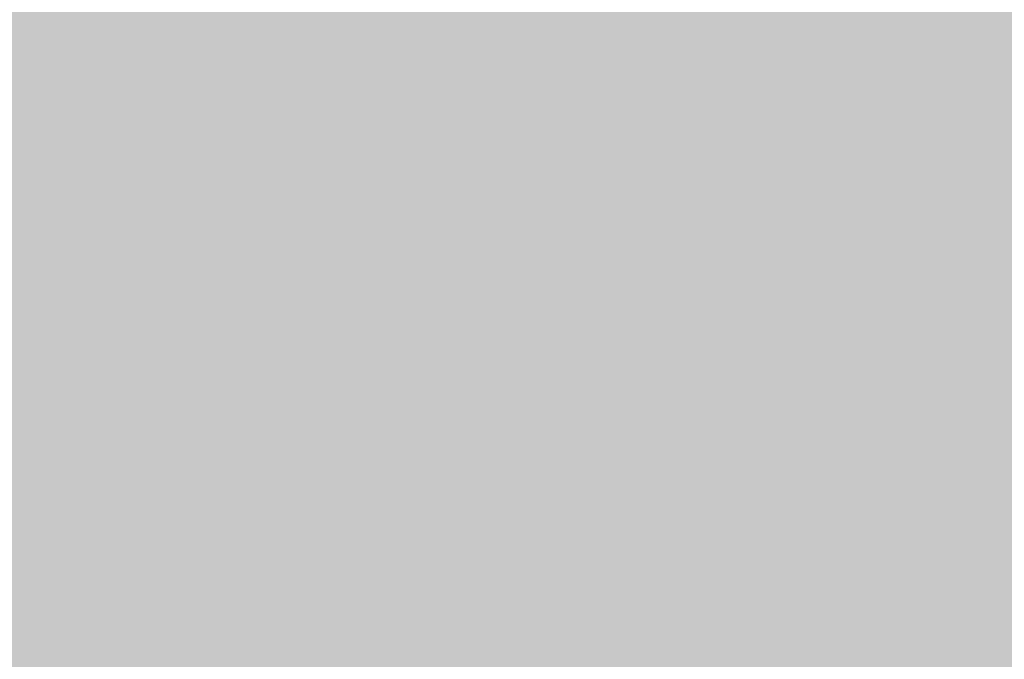
# Model space of a CAD drawing. Units: millimetres. Extents: x 0 to 2267, y 0 to 1823.
# Tile 135 of 256: x 1675 to 1760, y 1160 to 1216. Entities that reach past the tile are written whole.
import ezdxf

# ---------------------------------------------------------------- set-up
doc = ezdxf.new("R2010")
doc.units = ezdxf.units.MM
doc.header["$MEASUREMENT"] = 0
doc.layers.add('M-HATC', color=252, linetype='Continuous', lineweight=18)

msp = doc.modelspace()

# ---------------------------------------------------------------- hatches: boundary and pattern name
at = {"layer": 'M-HATC'}
h = msp.add_hatch(color=256, dxfattribs=at)
h.dxf.hatch_style = 1
h.paths.add_polyline_path([(2055.771, 1603.062), (1381.087, 1603.062), (1381.087, 1598.062), (2055.771, 1598.062)])
h.paths.add_polyline_path([(2055.771, 1598.062), (1381.087, 1598.062), (1381.087, 1593.062), (2055.771, 1593.062)])
h.paths.add_polyline_path([(2051.307, 1536.761), (1385.55, 1536.761), (1385.55, 1526.761), (1387.55, 1526.761), (1388.537, 1525.053), (1385.332, 1521.233), (1385.332, 1521.223), (2050.254, 1522.749), (2048.321, 1525.053), (2049.307, 1526.761), (2051.307, 1526.761)])
edge = h.paths.add_edge_path()
edge.add_arc((1847.535, 1379.149), 135, 222.60306, 222.89085, ccw=False)
edge.add_line((1748.166, 1287.766), (1683.092, 1287.766))
edge.add_arc((1583.724, 1379.149), 135, 317.10915, 317.39694, ccw=False)
edge.add_arc((1678.969, 1290.671), 5, 222.89085, 317.10915, ccw=False)
edge.add_arc((1774.213, 1379.149), 135, 222.60306, 222.89085, ccw=False)
edge.add_line((1674.845, 1287.766), (1609.771, 1287.766))
edge.add_arc((1510.403, 1379.149), 135, 317.10915, 317.39694, ccw=False)
edge.add_arc((1605.647, 1290.671), 5, 222.89085, 317.10915, ccw=False)
edge.add_arc((1700.892, 1379.149), 135, 222.60306, 222.89085, ccw=False)
edge.add_line((1601.524, 1287.766), (1536.45, 1287.766))
edge.add_arc((1437.081, 1379.149), 135, 317.10915, 317.39694, ccw=False)
edge.add_arc((1532.326, 1290.671), 5, 222.89085, 317.10915, ccw=False)
edge.add_arc((1627.571, 1379.149), 135, 222.60306, 222.89085, ccw=False)
edge.add_line((1528.203, 1287.766), (1505.929, 1287.766))
edge.add_spline(control_points=[(1505.929, 1287.766), (1504.262, 1287.766), (1504.262, 1282.766), (1505.929, 1282.766)], knot_values=[0, 0, 0, 0, 5, 5, 5, 5], degree=3, periodic=0)
edge.add_line((1505.929, 1282.766), (1930.929, 1282.766))
edge.add_spline(control_points=[(1930.929, 1282.766), (1932.596, 1282.766), (1932.596, 1287.766), (1930.929, 1287.766)], knot_values=[0, 0, 0, 0, 5, 5, 5, 5], degree=3, periodic=0)
edge.add_line((1930.929, 1287.766), (1903.056, 1287.766))
edge.add_arc((1803.688, 1379.149), 135, 317.10915, 317.39694, ccw=False)
edge.add_arc((1898.932, 1290.671), 5, 222.89085, 317.10915, ccw=False)
edge.add_arc((1994.177, 1379.149), 135, 222.60306, 222.89085, ccw=False)
edge.add_line((1894.809, 1287.766), (1829.735, 1287.766))
edge.add_arc((1730.366, 1379.149), 135, 317.10915, 317.39694, ccw=False)
edge.add_arc((1825.611, 1290.671), 5, 222.89085, 317.10915, ccw=False)
edge.add_arc((1920.856, 1379.149), 135, 222.60306, 222.89085, ccw=False)
edge.add_line((1821.487, 1287.766), (1756.413, 1287.766))
edge.add_arc((1657.045, 1379.149), 135, 317.10915, 317.39694, ccw=False)
edge.add_arc((1752.29, 1290.671), 5, 222.89085, 317.10915, ccw=False)
edge = h.paths.add_edge_path()
edge.add_spline(control_points=[(1843.429, 1227.247), (1845.096, 1227.247), (1845.096, 1232.247), (1843.429, 1232.247)], knot_values=[0, 0, 0, 0, 5, 5, 5, 5], degree=3, periodic=0)
edge.add_line((1843.429, 1232.247), (1593.429, 1232.247))
edge.add_spline(control_points=[(1593.429, 1232.247), (1591.762, 1232.247), (1591.762, 1227.247), (1593.429, 1227.247)], knot_values=[0, 0, 0, 0, 5, 5, 5, 5], degree=3, periodic=0)
edge.add_line((1593.429, 1227.247), (1843.429, 1227.247))
h.paths.add_polyline_path([(1905.929, 1127.417), (1530.929, 1127.417, 0.414214), (1520.929, 1117.417), (1530.929, 1117.417), (1915.929, 1117.417, 0.414214)])
edge = h.paths.add_edge_path()
edge.add_arc((1397.086, 1498.408), 12.73, 90.78215, 190.87871, ccw=False)
edge.add_line((1396.912, 1511.136), (1428.01, 1511.349))
edge.add_line((1428.01, 1511.349), (1433.01, 1511.349))
edge.add_line((1433.01, 1511.349), (1434.439, 1511.349))
edge.add_arc((1419.474, 1498.08), 20, 41.561, 74.08211)
edge.add_line((1424.959, 1517.314), (1399.935, 1517.256))
edge.add_spline(control_points=[(1399.931, 1517.256), (1399.884, 1517.213), (1399.833, 1517.169), (1399.777, 1517.124)], knot_values=[11.567499, 11.567499, 11.567499, 11.567499, 11.814249, 11.814249, 11.814249, 11.814249], degree=3, periodic=0)
edge.add_spline(control_points=[(1399.633, 1517.01), (1399.583, 1516.972), (1399.531, 1516.934), (1399.476, 1516.895)], knot_values=[11.167718, 11.167718, 11.167718, 11.167718, 11.365188, 11.365188, 11.365188, 11.365188], degree=3, periodic=0)
edge.add_spline(control_points=[(1399.34, 1516.8), (1399.151, 1516.672), (1398.938, 1516.538), (1398.704, 1516.399)], knot_values=[10.376405, 10.376405, 10.376405, 10.376405, 11.00994, 11.00994, 11.00994, 11.00994], degree=3, periodic=0)
edge.add_spline(control_points=[(1398.657, 1516.372), (1398.579, 1516.326), (1398.498, 1516.28), (1398.415, 1516.233)], knot_values=[10.125175, 10.125175, 10.125175, 10.125175, 10.334406, 10.334406, 10.334406, 10.334406], degree=3, periodic=0)
edge.add_spline(control_points=[(1398.264, 1516.149), (1398.196, 1516.111), (1398.126, 1516.073), (1398.055, 1516.035)], knot_values=[9.832246, 9.832246, 9.832246, 9.832246, 9.999658, 9.999658, 9.999658, 9.999658], degree=3, periodic=0)
edge.add_spline(control_points=[(1397.999, 1516.005), (1397.731, 1515.862), (1397.446, 1515.717), (1397.147, 1515.571)], knot_values=[9.161808, 9.161808, 9.161808, 9.161808, 9.787769, 9.787769, 9.787769, 9.787769], degree=3, periodic=0)
edge.add_spline(control_points=[(1397.147, 1515.571), (1396.842, 1515.423), (1396.522, 1515.274), (1396.191, 1515.126)], knot_values=[8.524455, 8.524455, 8.524455, 8.524455, 9.161808, 9.161808, 9.161808, 9.161808], degree=3, periodic=0)
edge.add_spline(control_points=[(1396.078, 1515.076), (1395.985, 1515.035), (1395.892, 1514.994), (1395.798, 1514.953)], knot_values=[8.275193, 8.275193, 8.275193, 8.275193, 8.451726, 8.451726, 8.451726, 8.451726], degree=3, periodic=0)
edge.add_spline(control_points=[(1395.602, 1514.869), (1395.5, 1514.826), (1395.397, 1514.782), (1395.293, 1514.739)], knot_values=[7.962917, 7.962917, 7.962917, 7.962917, 8.152764, 8.152764, 8.152764, 8.152764], degree=3, periodic=0)
edge.add_spline(control_points=[(1395.212, 1514.706), (1394.828, 1514.547), (1394.435, 1514.393), (1394.036, 1514.244)], knot_values=[7.21254, 7.21254, 7.21254, 7.21254, 7.913148, 7.913148, 7.913148, 7.913148], degree=3, periodic=0)
edge.add_spline(control_points=[(1394.036, 1514.244), (1393.708, 1514.121), (1393.375, 1514.003), (1393.043, 1513.889)], knot_values=[6.633733, 6.633733, 6.633733, 6.633733, 7.21254, 7.21254, 7.21254, 7.21254], degree=3, periodic=0)
edge.add_spline(control_points=[(1392.821, 1513.815), (1392.72, 1513.781), (1392.618, 1513.748), (1392.517, 1513.715)], knot_values=[6.328796, 6.328796, 6.328796, 6.328796, 6.505493, 6.505493, 6.505493, 6.505493], degree=3, periodic=0)
edge.add_spline(control_points=[(1392.517, 1513.715), (1392.319, 1513.652), (1392.121, 1513.59), (1391.924, 1513.531)], knot_values=[5.984605, 5.984605, 5.984605, 5.984605, 6.328796, 6.328796, 6.328796, 6.328796], degree=3, periodic=0)
edge.add_spline(control_points=[(1391.792, 1513.491), (1391.312, 1513.35), (1390.838, 1513.224), (1390.378, 1513.117)], knot_values=[5.066697, 5.066697, 5.066697, 5.066697, 5.907055, 5.907055, 5.907055, 5.907055], degree=3, periodic=0)
edge.add_spline(control_points=[(1390.378, 1513.117), (1390.18, 1513.071), (1389.984, 1513.028), (1389.791, 1512.99)], knot_values=[4.70367, 4.70367, 4.70367, 4.70367, 5.066695, 5.066695, 5.066695, 5.066695], degree=3, periodic=0)
edge.add_spline(control_points=[(1389.422, 1512.92), (1389.246, 1512.889), (1389.073, 1512.862), (1388.904, 1512.838)], knot_values=[4.130571, 4.130571, 4.130571, 4.130571, 4.469816, 4.469816, 4.469816, 4.469816], degree=3, periodic=0)
edge.add_spline(control_points=[(1388.904, 1512.838), (1388.591, 1512.795), (1388.291, 1512.764), (1388.007, 1512.749)], knot_values=[3.504031, 3.504031, 3.504031, 3.504031, 4.130571, 4.130571, 4.130571, 4.130571], degree=3, periodic=0)
edge.add_spline(control_points=[(1387.936, 1512.746), (1387.854, 1512.742), (1387.773, 1512.74), (1387.694, 1512.739)], knot_values=[3.268866, 3.268866, 3.268866, 3.268866, 3.451164, 3.451164, 3.451164, 3.451164], degree=3, periodic=0)
edge.add_spline(control_points=[(1387.335, 1512.744), (1387.208, 1512.75), (1387.085, 1512.76), (1386.967, 1512.774)], knot_values=[2.670686, 2.670686, 2.670686, 2.670686, 2.984, 2.984, 2.984, 2.984], degree=3, periodic=0)
edge.add_spline(control_points=[(1386.833, 1512.792), (1386.821, 1512.794), (1386.809, 1512.796), (1386.797, 1512.798)], knot_values=[2.516981, 2.516981, 2.516981, 2.516981, 2.549528, 2.549528, 2.549528, 2.549528], degree=3, periodic=0)
edge.add_spline(control_points=[(1386.453, 1512.873), (1386.426, 1512.881), (1386.399, 1512.889), (1386.373, 1512.897)], knot_values=[2.095869, 2.095869, 2.095869, 2.095869, 2.17941, 2.17941, 2.17941, 2.17941], degree=3, periodic=0)
edge.add_spline(control_points=[(1386.069, 1513.019), (1386.063, 1513.022), (1386.058, 1513.025), (1386.052, 1513.028)], knot_values=[1.72453, 1.72453, 1.72453, 1.72453, 1.745933, 1.745933, 1.745933, 1.745933], degree=3, periodic=0)
edge.add_arc((1399.474, 1498.08), 20, 131.82432, 180)
edge.add_arc((1630.334, 1505.548), 250.971, 181.70518, 236.42798)
edge.add_arc((1605.34, 1483.304), 218.782, 238.66083, 243.34961)
edge.add_arc((1647.091, 1510.359), 262.899, 183.12984, 237.85344, ccw=False)
h.paths.add_polyline_path([(1406.537, 1391.964, 0.149382), (1491.551, 1296.442, -0.129517)], flags=17)
edge = h.paths.add_edge_path()
edge.add_arc((2037.384, 1498.08), 20, 0, 48.26587)
edge.add_spline(control_points=[(2050.697, 1513.005), (2050.651, 1512.985), (2050.603, 1512.966), (2050.554, 1512.948)], knot_values=[1.835652, 1.835652, 1.835652, 1.835652, 2.000781, 2.000781, 2.000781, 2.000781], degree=3, periodic=0)
edge.add_spline(control_points=[(2050.462, 1512.917), (2050.479, 1512.922), (2050.496, 1512.928), (2050.513, 1512.934)], knot_values=[2.045477, 2.045477, 2.045477, 2.045477, 2.101389, 2.101389, 2.101389, 2.101389], degree=3, periodic=0)
edge.add_spline(control_points=[(2050.129, 1512.834), (2050.198, 1512.847), (2050.266, 1512.862), (2050.331, 1512.879)], knot_values=[2.237629, 2.237629, 2.237629, 2.237629, 2.435841, 2.435841, 2.435841, 2.435841], degree=3, periodic=0)
edge.add_spline(control_points=[(2050.095, 1512.828), (2050.106, 1512.83), (2050.118, 1512.832), (2050.129, 1512.834)], knot_values=[2.435841, 2.435841, 2.435841, 2.435841, 2.468321, 2.468321, 2.468321, 2.468321], degree=3, periodic=0)
edge.add_spline(control_points=[(2049.784, 1512.785), (2049.855, 1512.792), (2049.924, 1512.801), (2049.992, 1512.811)], knot_values=[2.563852, 2.563852, 2.563852, 2.563852, 2.748541, 2.748541, 2.748541, 2.748541], degree=3, periodic=0)
edge.add_spline(control_points=[(2049.405, 1512.762), (2049.536, 1512.765), (2049.663, 1512.773), (2049.784, 1512.785)], knot_values=[2.748541, 2.748541, 2.748541, 2.748541, 3.064882, 3.064882, 3.064882, 3.064882], degree=3, periodic=0)
edge.add_spline(control_points=[(2049.17, 1512.76), (2049.234, 1512.759), (2049.297, 1512.759), (2049.358, 1512.761)], knot_values=[3.102309, 3.102309, 3.102309, 3.102309, 3.2503, 3.2503, 3.2503, 3.2503], degree=3, periodic=0)
edge.add_spline(control_points=[(2048.857, 1512.769), (2048.964, 1512.764), (2049.068, 1512.761), (2049.17, 1512.76)], knot_values=[3.2503, 3.2503, 3.2503, 3.2503, 3.486069, 3.486069, 3.486069, 3.486069], degree=3, periodic=0)
edge.add_spline(control_points=[(2048.692, 1512.779), (2048.373, 1512.801), (2048.035, 1512.841), (2047.682, 1512.897)], knot_values=[3.606429, 3.606429, 3.606429, 3.606429, 4.2989, 4.2989, 4.2989, 4.2989], degree=3, periodic=0)
edge.add_spline(control_points=[(2047.682, 1512.897), (2047.546, 1512.919), (2047.408, 1512.942), (2047.268, 1512.969)], knot_values=[4.2989, 4.2989, 4.2989, 4.2989, 4.565769, 4.565769, 4.565769, 4.565769], degree=3, periodic=0)
edge.add_spline(control_points=[(2047.268, 1512.969), (2047.145, 1512.991), (2047.021, 1513.016), (2046.895, 1513.042)], knot_values=[4.565769, 4.565769, 4.565769, 4.565769, 4.799971, 4.799971, 4.799971, 4.799971], degree=3, periodic=0)
edge.add_spline(control_points=[(2046.895, 1513.042), (2046.529, 1513.119), (2046.151, 1513.209), (2045.768, 1513.311)], knot_values=[4.799971, 4.799971, 4.799971, 4.799971, 5.483718, 5.483718, 5.483718, 5.483718], degree=3, periodic=0)
edge.add_spline(control_points=[(2045.768, 1513.311), (2045.372, 1513.415), (2044.97, 1513.532), (2044.566, 1513.659)], knot_values=[5.483718, 5.483718, 5.483718, 5.483718, 6.187866, 6.187866, 6.187866, 6.187866], degree=3, periodic=0)
edge.add_spline(control_points=[(2044.566, 1513.659), (2044.415, 1513.706), (2044.263, 1513.755), (2044.112, 1513.805)], knot_values=[6.187866, 6.187866, 6.187866, 6.187866, 6.451551, 6.451551, 6.451551, 6.451551], degree=3, periodic=0)
edge.add_spline(control_points=[(2044.112, 1513.805), (2043.997, 1513.843), (2043.882, 1513.881), (2043.767, 1513.92)], knot_values=[6.451551, 6.451551, 6.451551, 6.451551, 6.651434, 6.651434, 6.651434, 6.651434], degree=3, periodic=0)
edge.add_spline(control_points=[(2043.767, 1513.92), (2043.372, 1514.055), (2042.977, 1514.198), (2042.589, 1514.346)], knot_values=[6.651434, 6.651434, 6.651434, 6.651434, 7.338879, 7.338879, 7.338879, 7.338879], degree=3, periodic=0)
edge.add_spline(control_points=[(2042.589, 1514.346), (2042.164, 1514.507), (2041.746, 1514.675), (2041.341, 1514.846)], knot_values=[7.338879, 7.338879, 7.338879, 7.338879, 8.089209, 8.089209, 8.089209, 8.089209], degree=3, periodic=0)
edge.add_spline(control_points=[(2041.341, 1514.846), (2041.103, 1514.946), (2040.869, 1515.048), (2040.64, 1515.15)], knot_values=[8.089209, 8.089209, 8.089209, 8.089209, 8.529587, 8.529587, 8.529587, 8.529587], degree=3, periodic=0)
edge.add_spline(control_points=[(2040.51, 1515.209), (2040.082, 1515.402), (2039.675, 1515.597), (2039.295, 1515.789)], knot_values=[8.613818, 8.613818, 8.613818, 8.613818, 9.44571, 9.44571, 9.44571, 9.44571], degree=3, periodic=0)
edge.add_spline(control_points=[(2039.295, 1515.789), (2039.062, 1515.907), (2038.839, 1516.025), (2038.629, 1516.14)], knot_values=[9.44571, 9.44571, 9.44571, 9.44571, 9.956404, 9.956404, 9.956404, 9.956404], degree=3, periodic=0)
edge.add_spline(control_points=[(2038.629, 1516.14), (2038.519, 1516.2), (2038.412, 1516.26), (2038.309, 1516.319)], knot_values=[9.956404, 9.956404, 9.956404, 9.956404, 10.223542, 10.223542, 10.223542, 10.223542], degree=3, periodic=0)
edge.add_spline(control_points=[(2038.309, 1516.319), (2038.214, 1516.374), (2038.122, 1516.428), (2038.033, 1516.481)], knot_values=[10.223542, 10.223542, 10.223542, 10.223542, 10.47051, 10.47051, 10.47051, 10.47051], degree=3, periodic=0)
edge.add_spline(control_points=[(2038.033, 1516.481), (2037.786, 1516.63), (2037.564, 1516.773), (2037.372, 1516.909)], knot_values=[10.47051, 10.47051, 10.47051, 10.47051, 11.15767, 11.15767, 11.15767, 11.15767], degree=3, periodic=0)
edge.add_spline(control_points=[(2037.372, 1516.909), (2037.279, 1516.975), (2037.193, 1517.04), (2037.114, 1517.102)], knot_values=[11.15767, 11.15767, 11.15767, 11.15767, 11.49227, 11.49227, 11.49227, 11.49227], degree=3, periodic=0)
edge.add_spline(control_points=[(2036.856, 1517.326), (2036.915, 1517.269), (2036.981, 1517.21), (2037.056, 1517.149)], knot_values=[11.577341, 11.577341, 11.577341, 11.577341, 11.91035, 11.91035, 11.91035, 11.91035], degree=3, periodic=0)
edge.add_spline(control_points=[(2036.807, 1517.375), (2036.823, 1517.359), (2036.839, 1517.342), (2036.856, 1517.326)], knot_values=[11.91035, 11.91035, 11.91035, 11.91035, 12.007402, 12.007402, 12.007402, 12.007402], degree=3, periodic=0)
edge.add_spline(control_points=[(2036.702, 1517.494), (2036.71, 1517.483), (2036.72, 1517.472), (2036.729, 1517.461)], knot_values=[12.184155, 12.184155, 12.184155, 12.184155, 12.255409, 12.255409, 12.255409, 12.255409], degree=3, periodic=0)
edge.add_spline(control_points=[(2036.616, 1517.621), (2036.62, 1517.613), (2036.624, 1517.606), (2036.629, 1517.598)], knot_values=[12.487913, 12.487913, 12.487913, 12.487913, 12.541035, 12.541035, 12.541035, 12.541035], degree=3, periodic=0)
edge.add_spline(control_points=[(2036.563, 1517.786), (2036.564, 1517.779), (2036.564, 1517.773), (2036.565, 1517.766)], knot_values=[12.911761, 12.911761, 12.911761, 12.911761, 12.968286, 12.968286, 12.968286, 12.968286], degree=3, periodic=0)
edge.add_spline(control_points=[(2036.617, 1517.93), (2036.612, 1517.926), (2036.609, 1517.921), (2036.605, 1517.916)], knot_values=[13.382527, 13.382527, 13.382527, 13.382527, 13.433791, 13.433791, 13.433791, 13.433791], degree=3, periodic=0)
edge.add_spline(control_points=[(2036.749, 1518.017), (2036.736, 1518.012), (2036.724, 1518.006), (2036.712, 1518)], knot_values=[13.726299, 13.726299, 13.726299, 13.726299, 13.809928, 13.809928, 13.809928, 13.809928], degree=3, periodic=0)
edge.add_spline(control_points=[(2036.86, 1518.053), (2036.839, 1518.047), (2036.818, 1518.042), (2036.799, 1518.035)], knot_values=[13.910887, 13.910887, 13.910887, 13.910887, 14.02153, 14.02153, 14.02153, 14.02153], degree=3, periodic=0)
edge.add_line((2036.964, 1518.08), (2032.384, 1518.08))
edge.add_line((2032.384, 1518.08), (2027.384, 1518.08))
edge.add_line((2027.384, 1518.08), (2022.384, 1518.08))
edge.add_line((2022.384, 1518.08), (2017.384, 1518.08))
edge.add_arc((2017.384, 1498.08), 20, 90, 138.439)
edge.add_line((2002.419, 1511.349), (2003.848, 1511.349))
edge.add_line((2003.848, 1511.349), (2008.848, 1511.349))
edge.add_line((2008.848, 1511.349), (2039.772, 1511.138))
edge.add_arc((2039.772, 1498.408), 12.73, -10.87871, 90, ccw=False)
edge.add_arc((1789.767, 1510.359), 262.899, 302.14656, 356.87016, ccw=False)
edge.add_arc((1831.518, 1483.304), 218.782, 296.65039, 301.33917)
edge.add_arc((1806.524, 1505.548), 250.971, 303.57202, 358.29482)
h.paths.add_polyline_path([(2030.321, 1391.964, -0.129517), (1945.307, 1296.442, 0.149382)], flags=17)
edge = h.paths.add_edge_path()
edge.add_spline(control_points=[(2037.246, 1518.082), (2037.29, 1518.081), (2037.336, 1518.08), (2037.384, 1518.08)], knot_values=[0.000012, 0.000012, 0.000012, 0.000012, 0.144754, 0.144754, 0.144754, 0.144754], degree=3, periodic=0)
edge.add_line((2037.336, 1518.08), (2037.01, 1518.08))
edge.add_spline(control_points=[(2037.01, 1518.08), (2036.982, 1518.077), (2036.956, 1518.073), (2036.931, 1518.068)], knot_values=[14.13465, 14.13465, 14.13465, 14.13465, 14.247197, 14.247197, 14.247197, 14.247197], degree=3, periodic=0)
edge.add_spline(control_points=[(2036.931, 1518.068), (2036.928, 1518.067), (2036.924, 1518.067), (2036.921, 1518.066)], knot_values=[14.118315, 14.118315, 14.118315, 14.118315, 14.13465, 14.13465, 14.13465, 14.13465], degree=3, periodic=0)
edge.add_spline(control_points=[(2036.921, 1518.066), (2036.912, 1518.064), (2036.903, 1518.063), (2036.895, 1518.061)], knot_values=[14.078086, 14.078086, 14.078086, 14.078086, 14.118315, 14.118315, 14.118315, 14.118315], degree=3, periodic=0)
edge.add_spline(control_points=[(2036.895, 1518.061), (2036.883, 1518.058), (2036.872, 1518.056), (2036.86, 1518.053)], knot_values=[14.02153, 14.02153, 14.02153, 14.02153, 14.078086, 14.078086, 14.078086, 14.078086], degree=3, periodic=0)
edge.add_spline(control_points=[(2036.86, 1518.053), (2036.839, 1518.047), (2036.818, 1518.042), (2036.799, 1518.035)], knot_values=[13.910887, 13.910887, 13.910887, 13.910887, 14.02153, 14.02153, 14.02153, 14.02153], degree=3, periodic=0)
edge.add_spline(control_points=[(2036.799, 1518.035), (2036.798, 1518.035), (2036.797, 1518.035), (2036.797, 1518.035)], knot_values=[13.906906, 13.906906, 13.906906, 13.906906, 13.910887, 13.910887, 13.910887, 13.910887], degree=3, periodic=0)
edge.add_spline(control_points=[(2036.797, 1518.035), (2036.788, 1518.032), (2036.78, 1518.029), (2036.772, 1518.026)], knot_values=[13.857826, 13.857826, 13.857826, 13.857826, 13.906906, 13.906906, 13.906906, 13.906906], degree=3, periodic=0)
edge.add_spline(control_points=[(2036.772, 1518.026), (2036.764, 1518.023), (2036.756, 1518.02), (2036.749, 1518.017)], knot_values=[13.809928, 13.809928, 13.809928, 13.809928, 13.857826, 13.857826, 13.857826, 13.857826], degree=3, periodic=0)
edge.add_spline(control_points=[(2036.749, 1518.017), (2036.736, 1518.012), (2036.724, 1518.006), (2036.712, 1518)], knot_values=[13.726299, 13.726299, 13.726299, 13.726299, 13.809928, 13.809928, 13.809928, 13.809928], degree=3, periodic=0)
edge.add_spline(control_points=[(2036.712, 1518), (2036.712, 1518), (2036.712, 1518), (2036.711, 1518)], knot_values=[13.723993, 13.723993, 13.723993, 13.723993, 13.726299, 13.726299, 13.726299, 13.726299], degree=3, periodic=0)
edge.add_spline(control_points=[(2036.711, 1518), (2036.706, 1517.997), (2036.701, 1517.994), (2036.696, 1517.992)], knot_values=[13.686536, 13.686536, 13.686536, 13.686536, 13.723993, 13.723993, 13.723993, 13.723993], degree=3, periodic=0)
edge.add_spline(control_points=[(2036.696, 1517.992), (2036.692, 1517.989), (2036.687, 1517.987), (2036.683, 1517.984)], knot_values=[13.651251, 13.651251, 13.651251, 13.651251, 13.686536, 13.686536, 13.686536, 13.686536], degree=3, periodic=0)
edge.add_spline(control_points=[(2036.683, 1517.984), (2036.676, 1517.98), (2036.67, 1517.976), (2036.664, 1517.971)], knot_values=[13.596804, 13.596804, 13.596804, 13.596804, 13.651251, 13.651251, 13.651251, 13.651251], degree=3, periodic=0)
edge.add_spline(control_points=[(2036.664, 1517.971), (2036.664, 1517.971), (2036.663, 1517.971), (2036.663, 1517.971)], knot_values=[13.593956, 13.593956, 13.593956, 13.593956, 13.596804, 13.596804, 13.596804, 13.596804], degree=3, periodic=0)
edge.add_spline(control_points=[(2036.663, 1517.971), (2036.66, 1517.969), (2036.658, 1517.967), (2036.655, 1517.965)], knot_values=[13.570322, 13.570322, 13.570322, 13.570322, 13.593956, 13.593956, 13.593956, 13.593956], degree=3, periodic=0)
edge.add_spline(control_points=[(2036.655, 1517.965), (2036.653, 1517.963), (2036.65, 1517.961), (2036.647, 1517.959)], knot_values=[13.545477, 13.545477, 13.545477, 13.545477, 13.570322, 13.570322, 13.570322, 13.570322], degree=3, periodic=0)
edge.add_spline(control_points=[(2036.647, 1517.959), (2036.647, 1517.959), (2036.647, 1517.959), (2036.647, 1517.959)], knot_values=[13.543931, 13.543931, 13.543931, 13.543931, 13.545477, 13.545477, 13.545477, 13.545477], degree=3, periodic=0)
edge.add_spline(control_points=[(2036.647, 1517.959), (2036.641, 1517.954), (2036.636, 1517.949), (2036.631, 1517.945)], knot_values=[13.488237, 13.488237, 13.488237, 13.488237, 13.543931, 13.543931, 13.543931, 13.543931], degree=3, periodic=0)
edge.add_spline(control_points=[(2036.631, 1517.945), (2036.628, 1517.942), (2036.626, 1517.94), (2036.623, 1517.937)], knot_values=[13.460307, 13.460307, 13.460307, 13.460307, 13.488237, 13.488237, 13.488237, 13.488237], degree=3, periodic=0)
edge.add_spline(control_points=[(2036.623, 1517.937), (2036.622, 1517.936), (2036.62, 1517.934), (2036.618, 1517.932)], knot_values=[13.439712, 13.439712, 13.439712, 13.439712, 13.460307, 13.460307, 13.460307, 13.460307], degree=3, periodic=0)
edge.add_spline(control_points=[(2036.618, 1517.932), (2036.618, 1517.931), (2036.617, 1517.931), (2036.617, 1517.93)], knot_values=[13.433791, 13.433791, 13.433791, 13.433791, 13.439712, 13.439712, 13.439712, 13.439712], degree=3, periodic=0)
edge.add_spline(control_points=[(2036.617, 1517.93), (2036.612, 1517.926), (2036.609, 1517.921), (2036.605, 1517.916)], knot_values=[13.382527, 13.382527, 13.382527, 13.382527, 13.433791, 13.433791, 13.433791, 13.433791], degree=3, periodic=0)
edge.add_spline(control_points=[(2036.605, 1517.916), (2036.603, 1517.913), (2036.6, 1517.91), (2036.598, 1517.907)], knot_values=[13.350017, 13.350017, 13.350017, 13.350017, 13.382527, 13.382527, 13.382527, 13.382527], degree=3, periodic=0)
edge.add_spline(control_points=[(2036.598, 1517.907), (2036.597, 1517.906), (2036.596, 1517.904), (2036.595, 1517.903)], knot_values=[13.333922, 13.333922, 13.333922, 13.333922, 13.350017, 13.350017, 13.350017, 13.350017], degree=3, periodic=0)
edge.add_spline(control_points=[(2036.595, 1517.903), (2036.595, 1517.902), (2036.594, 1517.901), (2036.593, 1517.9)], knot_values=[13.323828, 13.323828, 13.323828, 13.323828, 13.333922, 13.333922, 13.333922, 13.333922], degree=3, periodic=0)
edge.add_spline(control_points=[(2036.593, 1517.9), (2036.59, 1517.895), (2036.588, 1517.891), (2036.585, 1517.886)], knot_values=[13.277545, 13.277545, 13.277545, 13.277545, 13.323828, 13.323828, 13.323828, 13.323828], degree=3, periodic=0)
edge.add_spline(control_points=[(2036.585, 1517.886), (2036.584, 1517.883), (2036.582, 1517.879), (2036.58, 1517.875)], knot_values=[13.240119, 13.240119, 13.240119, 13.240119, 13.277545, 13.277545, 13.277545, 13.277545], degree=3, periodic=0)
edge.add_spline(control_points=[(2036.58, 1517.875), (2036.58, 1517.874), (2036.579, 1517.873), (2036.578, 1517.872)], knot_values=[13.228211, 13.228211, 13.228211, 13.228211, 13.240119, 13.240119, 13.240119, 13.240119], degree=3, periodic=0)
edge.add_spline(control_points=[(2036.578, 1517.872), (2036.578, 1517.87), (2036.577, 1517.869), (2036.577, 1517.868)], knot_values=[13.215717, 13.215717, 13.215717, 13.215717, 13.228211, 13.228211, 13.228211, 13.228211], degree=3, periodic=0)
edge.add_spline(control_points=[(2036.577, 1517.868), (2036.575, 1517.864), (2036.574, 1517.86), (2036.573, 1517.857)], knot_values=[13.179847, 13.179847, 13.179847, 13.179847, 13.215717, 13.215717, 13.215717, 13.215717], degree=3, periodic=0)
edge.add_spline(control_points=[(2036.573, 1517.857), (2036.571, 1517.851), (2036.57, 1517.846), (2036.569, 1517.841)], knot_values=[13.132017, 13.132017, 13.132017, 13.132017, 13.179847, 13.179847, 13.179847, 13.179847], degree=3, periodic=0)
edge.add_spline(control_points=[(2036.569, 1517.841), (2036.568, 1517.84), (2036.568, 1517.839), (2036.568, 1517.838)], knot_values=[13.122482, 13.122482, 13.122482, 13.122482, 13.132017, 13.132017, 13.132017, 13.132017], degree=3, periodic=0)
edge.add_spline(control_points=[(2036.568, 1517.838), (2036.568, 1517.836), (2036.567, 1517.835), (2036.567, 1517.833)], knot_values=[13.105592, 13.105592, 13.105592, 13.105592, 13.122482, 13.122482, 13.122482, 13.122482], degree=3, periodic=0)
edge.add_spline(control_points=[(2036.567, 1517.833), (2036.566, 1517.829), (2036.566, 1517.826), (2036.565, 1517.822)], knot_values=[13.074063, 13.074063, 13.074063, 13.074063, 13.105592, 13.105592, 13.105592, 13.105592], degree=3, periodic=0)
edge.add_spline(control_points=[(2036.565, 1517.822), (2036.565, 1517.822), (2036.565, 1517.822), (2036.565, 1517.822)], knot_values=[13.074043, 13.074043, 13.074043, 13.074043, 13.074063, 13.074063, 13.074063, 13.074063], degree=3, periodic=0)
edge.add_spline(control_points=[(2036.565, 1517.822), (2036.564, 1517.816), (2036.564, 1517.811), (2036.564, 1517.805)], knot_values=[13.021884, 13.021884, 13.021884, 13.021884, 13.074043, 13.074043, 13.074043, 13.074043], degree=3, periodic=0)
edge.add_spline(control_points=[(2036.564, 1517.805), (2036.564, 1517.804), (2036.564, 1517.803), (2036.564, 1517.803)], knot_values=[13.01674, 13.01674, 13.01674, 13.01674, 13.021884, 13.021884, 13.021884, 13.021884], degree=3, periodic=0)
edge.add_spline(control_points=[(2036.564, 1517.803), (2036.563, 1517.801), (2036.563, 1517.798), (2036.563, 1517.796)], knot_values=[12.996438, 12.996438, 12.996438, 12.996438, 13.01674, 13.01674, 13.01674, 13.01674], degree=3, periodic=0)
edge.add_spline(control_points=[(2036.563, 1517.796), (2036.563, 1517.793), (2036.563, 1517.789), (2036.563, 1517.786)], knot_values=[12.968286, 12.968286, 12.968286, 12.968286, 12.996438, 12.996438, 12.996438, 12.996438], degree=3, periodic=0)
edge.add_spline(control_points=[(2036.563, 1517.786), (2036.564, 1517.779), (2036.564, 1517.773), (2036.565, 1517.766)], knot_values=[12.911761, 12.911761, 12.911761, 12.911761, 12.968286, 12.968286, 12.968286, 12.968286], degree=3, periodic=0)
edge.add_spline(control_points=[(2036.565, 1517.766), (2036.565, 1517.766), (2036.565, 1517.766), (2036.565, 1517.766)], knot_values=[12.911017, 12.911017, 12.911017, 12.911017, 12.911761, 12.911761, 12.911761, 12.911761], degree=3, periodic=0)
edge.add_spline(control_points=[(2036.565, 1517.766), (2036.565, 1517.762), (2036.566, 1517.759), (2036.566, 1517.756)], knot_values=[12.88528, 12.88528, 12.88528, 12.88528, 12.911017, 12.911017, 12.911017, 12.911017], degree=3, periodic=0)
edge.add_spline(control_points=[(2036.566, 1517.756), (2036.567, 1517.753), (2036.567, 1517.751), (2036.568, 1517.748)], knot_values=[12.862519, 12.862519, 12.862519, 12.862519, 12.88528, 12.88528, 12.88528, 12.88528], degree=3, periodic=0)
edge.add_spline(control_points=[(2036.568, 1517.748), (2036.568, 1517.747), (2036.568, 1517.747), (2036.568, 1517.746)], knot_values=[12.858885, 12.858885, 12.858885, 12.858885, 12.862519, 12.862519, 12.862519, 12.862519], degree=3, periodic=0)
edge.add_spline(control_points=[(2036.568, 1517.746), (2036.569, 1517.74), (2036.571, 1517.733), (2036.572, 1517.726)], knot_values=[12.8053, 12.8053, 12.8053, 12.8053, 12.858885, 12.858885, 12.858885, 12.858885], degree=3, periodic=0)
edge.add_spline(control_points=[(2036.572, 1517.726), (2036.573, 1517.723), (2036.574, 1517.719), (2036.576, 1517.715)], knot_values=[12.775176, 12.775176, 12.775176, 12.775176, 12.8053, 12.8053, 12.8053, 12.8053], degree=3, periodic=0)
edge.add_spline(control_points=[(2036.576, 1517.715), (2036.576, 1517.713), (2036.577, 1517.71), (2036.578, 1517.708)], knot_values=[12.756759, 12.756759, 12.756759, 12.756759, 12.775176, 12.775176, 12.775176, 12.775176], degree=3, periodic=0)
edge.add_spline(control_points=[(2036.578, 1517.708), (2036.578, 1517.707), (2036.578, 1517.706), (2036.579, 1517.705)], knot_values=[12.748742, 12.748742, 12.748742, 12.748742, 12.756759, 12.756759, 12.756759, 12.756759], degree=3, periodic=0)
edge.add_spline(control_points=[(2036.579, 1517.705), (2036.581, 1517.698), (2036.583, 1517.692), (2036.586, 1517.685)], knot_values=[12.69959, 12.69959, 12.69959, 12.69959, 12.748742, 12.748742, 12.748742, 12.748742], degree=3, periodic=0)
edge.add_spline(control_points=[(2036.586, 1517.685), (2036.588, 1517.68), (2036.59, 1517.675), (2036.592, 1517.669)], knot_values=[12.659038, 12.659038, 12.659038, 12.659038, 12.69959, 12.69959, 12.69959, 12.69959], degree=3, periodic=0)
edge.add_spline(control_points=[(2036.592, 1517.669), (2036.594, 1517.665), (2036.596, 1517.66), (2036.598, 1517.656)], knot_values=[12.626806, 12.626806, 12.626806, 12.626806, 12.659038, 12.659038, 12.659038, 12.659038], degree=3, periodic=0)
edge.add_spline(control_points=[(2036.598, 1517.656), (2036.598, 1517.655), (2036.599, 1517.654), (2036.599, 1517.653)], knot_values=[12.619394, 12.619394, 12.619394, 12.619394, 12.626806, 12.626806, 12.626806, 12.626806], degree=3, periodic=0)
edge.add_spline(control_points=[(2036.599, 1517.653), (2036.604, 1517.642), (2036.61, 1517.632), (2036.616, 1517.621)], knot_values=[12.541039, 12.541039, 12.541039, 12.541039, 12.619394, 12.619394, 12.619394, 12.619394], degree=3, periodic=0)
edge.add_spline(control_points=[(2036.616, 1517.621), (2036.616, 1517.621), (2036.616, 1517.621), (2036.616, 1517.621)], knot_values=[12.541035, 12.541035, 12.541035, 12.541035, 12.541039, 12.541039, 12.541039, 12.541039], degree=3, periodic=0)
edge.add_spline(control_points=[(2036.616, 1517.621), (2036.62, 1517.613), (2036.624, 1517.606), (2036.629, 1517.598)], knot_values=[12.487913, 12.487913, 12.487913, 12.487913, 12.541035, 12.541035, 12.541035, 12.541035], degree=3, periodic=0)
edge.add_spline(control_points=[(2036.629, 1517.598), (2036.633, 1517.592), (2036.637, 1517.585), (2036.641, 1517.579)], knot_values=[12.443982, 12.443982, 12.443982, 12.443982, 12.487913, 12.487913, 12.487913, 12.487913], degree=3, periodic=0)
edge.add_spline(control_points=[(2036.641, 1517.579), (2036.641, 1517.578), (2036.642, 1517.576), (2036.643, 1517.575)], knot_values=[12.434996, 12.434996, 12.434996, 12.434996, 12.443982, 12.443982, 12.443982, 12.443982], degree=3, periodic=0)
edge.add_spline(control_points=[(2036.643, 1517.575), (2036.653, 1517.56), (2036.664, 1517.544), (2036.676, 1517.528)], knot_values=[12.329647, 12.329647, 12.329647, 12.329647, 12.434996, 12.434996, 12.434996, 12.434996], degree=3, periodic=0)
edge.add_spline(control_points=[(2036.676, 1517.528), (2036.684, 1517.517), (2036.693, 1517.505), (2036.702, 1517.494)], knot_values=[12.255409, 12.255409, 12.255409, 12.255409, 12.329647, 12.329647, 12.329647, 12.329647], degree=3, periodic=0)
edge.add_spline(control_points=[(2036.702, 1517.494), (2036.71, 1517.483), (2036.72, 1517.472), (2036.729, 1517.461)], knot_values=[12.184155, 12.184155, 12.184155, 12.184155, 12.255409, 12.255409, 12.255409, 12.255409], degree=3, periodic=0)
edge.add_spline(control_points=[(2036.729, 1517.461), (2036.744, 1517.444), (2036.759, 1517.426), (2036.775, 1517.409)], knot_values=[12.075961, 12.075961, 12.075961, 12.075961, 12.184155, 12.184155, 12.184155, 12.184155], degree=3, periodic=0)
edge.add_spline(control_points=[(2036.775, 1517.409), (2036.776, 1517.407), (2036.777, 1517.406), (2036.778, 1517.405)], knot_values=[12.069502, 12.069502, 12.069502, 12.069502, 12.075961, 12.075961, 12.075961, 12.075961], degree=3, periodic=0)
edge.add_spline(control_points=[(2036.778, 1517.405), (2036.788, 1517.395), (2036.797, 1517.385), (2036.807, 1517.375)], knot_values=[12.007402, 12.007402, 12.007402, 12.007402, 12.069502, 12.069502, 12.069502, 12.069502], degree=3, periodic=0)
edge.add_spline(control_points=[(2036.807, 1517.375), (2036.823, 1517.359), (2036.839, 1517.342), (2036.856, 1517.326)], knot_values=[11.91035, 11.91035, 11.91035, 11.91035, 12.007402, 12.007402, 12.007402, 12.007402], degree=3, periodic=0)
edge.add_spline(control_points=[(2036.856, 1517.326), (2036.915, 1517.269), (2036.981, 1517.21), (2037.056, 1517.149)], knot_values=[11.577341, 11.577341, 11.577341, 11.577341, 11.91035, 11.91035, 11.91035, 11.91035], degree=3, periodic=0)
edge.add_spline(control_points=[(2037.056, 1517.149), (2037.075, 1517.134), (2037.094, 1517.118), (2037.114, 1517.102)], knot_values=[11.49227, 11.49227, 11.49227, 11.49227, 11.577341, 11.577341, 11.577341, 11.577341], degree=3, periodic=0)
edge.add_spline(control_points=[(2037.114, 1517.102), (2037.193, 1517.04), (2037.279, 1516.975), (2037.372, 1516.909)], knot_values=[11.15767, 11.15767, 11.15767, 11.15767, 11.49227, 11.49227, 11.49227, 11.49227], degree=3, periodic=0)
edge.add_spline(control_points=[(2037.372, 1516.909), (2037.564, 1516.773), (2037.786, 1516.63), (2038.033, 1516.481)], knot_values=[10.47051, 10.47051, 10.47051, 10.47051, 11.15767, 11.15767, 11.15767, 11.15767], degree=3, periodic=0)
edge.add_spline(control_points=[(2038.033, 1516.481), (2038.122, 1516.428), (2038.214, 1516.374), (2038.309, 1516.319)], knot_values=[10.223542, 10.223542, 10.223542, 10.223542, 10.47051, 10.47051, 10.47051, 10.47051], degree=3, periodic=0)
edge.add_spline(control_points=[(2038.309, 1516.319), (2038.412, 1516.26), (2038.519, 1516.2), (2038.629, 1516.14)], knot_values=[9.956404, 9.956404, 9.956404, 9.956404, 10.223542, 10.223542, 10.223542, 10.223542], degree=3, periodic=0)
edge.add_spline(control_points=[(2038.629, 1516.14), (2038.839, 1516.025), (2039.062, 1515.907), (2039.295, 1515.789)], knot_values=[9.44571, 9.44571, 9.44571, 9.44571, 9.956404, 9.956404, 9.956404, 9.956404], degree=3, periodic=0)
edge.add_spline(control_points=[(2039.295, 1515.789), (2039.675, 1515.597), (2040.082, 1515.402), (2040.51, 1515.209)], knot_values=[8.613818, 8.613818, 8.613818, 8.613818, 9.44571, 9.44571, 9.44571, 9.44571], degree=3, periodic=0)
edge.add_spline(control_points=[(2040.51, 1515.209), (2040.553, 1515.189), (2040.597, 1515.17), (2040.64, 1515.15)], knot_values=[8.529587, 8.529587, 8.529587, 8.529587, 8.613818, 8.613818, 8.613818, 8.613818], degree=3, periodic=0)
edge.add_spline(control_points=[(2040.64, 1515.15), (2040.869, 1515.048), (2041.103, 1514.946), (2041.341, 1514.846)], knot_values=[8.089209, 8.089209, 8.089209, 8.089209, 8.529587, 8.529587, 8.529587, 8.529587], degree=3, periodic=0)
edge.add_spline(control_points=[(2041.341, 1514.846), (2041.746, 1514.675), (2042.164, 1514.507), (2042.589, 1514.346)], knot_values=[7.338879, 7.338879, 7.338879, 7.338879, 8.089209, 8.089209, 8.089209, 8.089209], degree=3, periodic=0)
edge.add_spline(control_points=[(2042.589, 1514.346), (2042.977, 1514.198), (2043.372, 1514.055), (2043.767, 1513.92)], knot_values=[6.651434, 6.651434, 6.651434, 6.651434, 7.338879, 7.338879, 7.338879, 7.338879], degree=3, periodic=0)
edge.add_spline(control_points=[(2043.767, 1513.92), (2043.882, 1513.881), (2043.997, 1513.843), (2044.112, 1513.805)], knot_values=[6.451551, 6.451551, 6.451551, 6.451551, 6.651434, 6.651434, 6.651434, 6.651434], degree=3, periodic=0)
edge.add_spline(control_points=[(2044.112, 1513.805), (2044.263, 1513.755), (2044.415, 1513.706), (2044.566, 1513.659)], knot_values=[6.187866, 6.187866, 6.187866, 6.187866, 6.451551, 6.451551, 6.451551, 6.451551], degree=3, periodic=0)
edge.add_spline(control_points=[(2044.566, 1513.659), (2044.97, 1513.532), (2045.372, 1513.415), (2045.768, 1513.311)], knot_values=[5.483718, 5.483718, 5.483718, 5.483718, 6.187866, 6.187866, 6.187866, 6.187866], degree=3, periodic=0)
edge.add_spline(control_points=[(2045.768, 1513.311), (2046.151, 1513.209), (2046.529, 1513.119), (2046.895, 1513.042)], knot_values=[4.799971, 4.799971, 4.799971, 4.799971, 5.483718, 5.483718, 5.483718, 5.483718], degree=3, periodic=0)
edge.add_spline(control_points=[(2046.895, 1513.042), (2047.021, 1513.016), (2047.145, 1512.991), (2047.268, 1512.969)], knot_values=[4.565769, 4.565769, 4.565769, 4.565769, 4.799971, 4.799971, 4.799971, 4.799971], degree=3, periodic=0)
edge.add_spline(control_points=[(2047.268, 1512.969), (2047.408, 1512.942), (2047.546, 1512.919), (2047.682, 1512.897)], knot_values=[4.2989, 4.2989, 4.2989, 4.2989, 4.565769, 4.565769, 4.565769, 4.565769], degree=3, periodic=0)
edge.add_spline(control_points=[(2047.682, 1512.897), (2048.035, 1512.841), (2048.373, 1512.801), (2048.692, 1512.779)], knot_values=[3.606429, 3.606429, 3.606429, 3.606429, 4.2989, 4.2989, 4.2989, 4.2989], degree=3, periodic=0)
edge.add_spline(control_points=[(2048.692, 1512.779), (2048.748, 1512.775), (2048.803, 1512.772), (2048.857, 1512.769)], knot_values=[3.486069, 3.486069, 3.486069, 3.486069, 3.606429, 3.606429, 3.606429, 3.606429], degree=3, periodic=0)
edge.add_spline(control_points=[(2048.857, 1512.769), (2048.964, 1512.764), (2049.068, 1512.761), (2049.17, 1512.76)], knot_values=[3.2503, 3.2503, 3.2503, 3.2503, 3.486069, 3.486069, 3.486069, 3.486069], degree=3, periodic=0)
edge.add_spline(control_points=[(2049.17, 1512.76), (2049.234, 1512.759), (2049.297, 1512.759), (2049.358, 1512.761)], knot_values=[3.102309, 3.102309, 3.102309, 3.102309, 3.2503, 3.2503, 3.2503, 3.2503], degree=3, periodic=0)
edge.add_spline(control_points=[(2049.358, 1512.761), (2049.374, 1512.761), (2049.39, 1512.761), (2049.405, 1512.762)], knot_values=[3.064882, 3.064882, 3.064882, 3.064882, 3.102309, 3.102309, 3.102309, 3.102309], degree=3, periodic=0)
edge.add_spline(control_points=[(2049.405, 1512.762), (2049.536, 1512.765), (2049.663, 1512.773), (2049.784, 1512.785)], knot_values=[2.748541, 2.748541, 2.748541, 2.748541, 3.064882, 3.064882, 3.064882, 3.064882], degree=3, periodic=0)
edge.add_spline(control_points=[(2049.784, 1512.785), (2049.855, 1512.792), (2049.924, 1512.801), (2049.992, 1512.811)], knot_values=[2.563852, 2.563852, 2.563852, 2.563852, 2.748541, 2.748541, 2.748541, 2.748541], degree=3, periodic=0)
edge.add_spline(control_points=[(2049.992, 1512.811), (2050.026, 1512.816), (2050.061, 1512.822), (2050.095, 1512.828)], knot_values=[2.468321, 2.468321, 2.468321, 2.468321, 2.563852, 2.563852, 2.563852, 2.563852], degree=3, periodic=0)
edge.add_spline(control_points=[(2050.095, 1512.828), (2050.106, 1512.83), (2050.118, 1512.832), (2050.129, 1512.834)], knot_values=[2.435841, 2.435841, 2.435841, 2.435841, 2.468321, 2.468321, 2.468321, 2.468321], degree=3, periodic=0)
edge.add_spline(control_points=[(2050.129, 1512.834), (2050.198, 1512.847), (2050.266, 1512.862), (2050.331, 1512.879)], knot_values=[2.237629, 2.237629, 2.237629, 2.237629, 2.435841, 2.435841, 2.435841, 2.435841], degree=3, periodic=0)
edge.add_spline(control_points=[(2050.331, 1512.879), (2050.375, 1512.891), (2050.419, 1512.903), (2050.462, 1512.917)], knot_values=[2.101389, 2.101389, 2.101389, 2.101389, 2.237629, 2.237629, 2.237629, 2.237629], degree=3, periodic=0)
edge.add_spline(control_points=[(2050.462, 1512.917), (2050.479, 1512.922), (2050.496, 1512.928), (2050.513, 1512.934)], knot_values=[2.045477, 2.045477, 2.045477, 2.045477, 2.101389, 2.101389, 2.101389, 2.101389], degree=3, periodic=0)
edge.add_spline(control_points=[(2050.513, 1512.934), (2050.527, 1512.938), (2050.54, 1512.943), (2050.554, 1512.948)], knot_values=[2.000781, 2.000781, 2.000781, 2.000781, 2.045477, 2.045477, 2.045477, 2.045477], degree=3, periodic=0)
edge.add_spline(control_points=[(2050.554, 1512.948), (2050.603, 1512.966), (2050.651, 1512.985), (2050.697, 1513.005)], knot_values=[1.835652, 1.835652, 1.835652, 1.835652, 2.000781, 2.000781, 2.000781, 2.000781], degree=3, periodic=0)
edge.add_arc((2037.384, 1498.08), 20, 48.26587, 90.12993)
edge = h.paths.add_edge_path(flags=16)
edge.add_spline(control_points=[(1386.139, 1512.986), (1388.92, 1511.739), (1398.039, 1515.519), (1399.931, 1517.256)], knot_values=[1.831046, 1.831046, 1.831046, 1.831046, 11.814249, 11.814249, 11.814249, 11.814249], degree=3, periodic=0)
edge.add_line((1399.931, 1517.256), (1393.743, 1517.242))
edge.add_arc((1399.474, 1498.08), 20, 106.6501, 131.8173)
h = msp.add_hatch(color=256, dxfattribs=at)
h.dxf.hatch_style = 1
h.paths.add_polyline_path([(2042.889, 1580.18), (2055.771, 1593.062), (1381.087, 1593.062), (1393.969, 1580.18), (1374.086, 1560.296), (2062.772, 1560.296)])
h.paths.add_polyline_path([(1843.429, 1201.33), (1843.429, 1227.247), (1593.429, 1227.247), (1593.429, 1201.33, -0.228274), (1574.599, 1162.235), (1530.929, 1127.417), (1905.929, 1127.417), (1862.259, 1162.235, -0.228274)])

doc.saveas('drawing.dxf')
